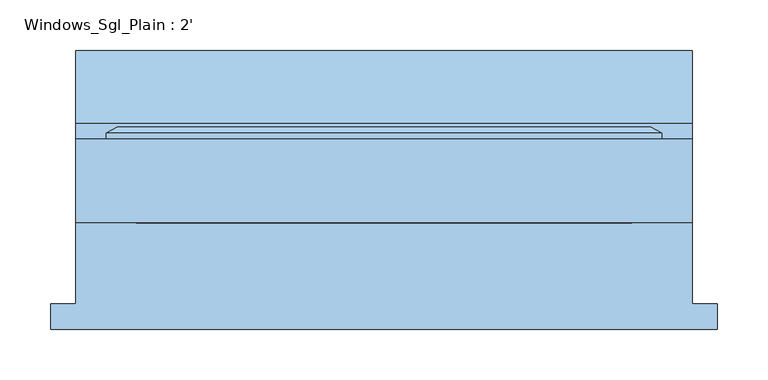
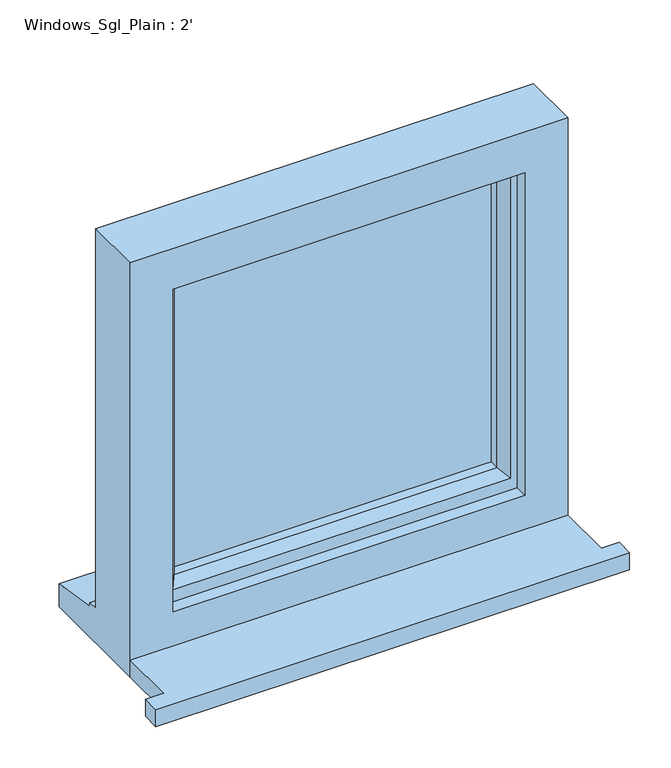
"""IFC4 building model written with IfcOpenShell, lengths in millimetres: window geometry, Windows_Sgl_Plain : 2'."""

from ifc_helpers import new_model, si_unit, frame, origin, place, context, project, spatial, polyline, outline, extrude, faceted_brep, source, transform, mapped, element, save


def windows_sgl_plain_2_298b83e7(model_context):
    return source(origin(), model_context, "Body", "SolidModel", [
        extrude(outline(polyline([(-329.8, -123.2234322), (-329.8, -98.2234322), (-304.8, -98.2234322), (-304.8, -17.8634322), (304.8, -17.8634322), (304.8, -98.2234322), (329.8, -98.2234322), (329.8, -123.2234322), (-329.8, -123.2234322)])), frame((0.0, 0.0, 1500.4), z_axis=(0.0, 0.0, 1.0), x_axis=(1.0, 0.0, 0.0)), (0.0, 0.0, 1.0), 25.0),
        faceted_brep([(-304.8, -17.8634322, 1500.4), (304.8, -17.8634322, 1500.4), (304.8, -17.8634322, 2110.0), (-304.8, -17.8634322, 2110.0), (-244.8, -17.8634322, 2050.0), (244.8, -17.8634322, 2050.0), (244.8, -17.8634322, 1575.4), (-244.8, -17.8634322, 1575.4), (-304.8, 65.1365678, 2110.0), (-304.8, 65.1365678, 1551.4), (-304.8, 80.1365678, 1550.08767), (-304.8, 80.1365678, 1545.1449676), (-304.8, 152.6365678, 1534.2088847), (-304.8, 152.6365678, 1500.4), (304.8, 65.1365678, 2110.0), (304.8, 65.1365678, 1551.4), (-264.8, 65.1365678, 2070.0), (-264.8, 65.1365678, 1563.4), (264.8, 65.1365678, 1563.4), (264.8, 65.1365678, 2070.0), (-264.8, 0.1365678, 2070.0), (-264.8, 0.1365678, 1563.4), (264.8, 0.1365678, 2070.0), (264.8, 0.1365678, 1563.4), (-244.8, 0.1365678, 2050.0), (-244.8, 0.1365678, 1575.4), (244.8, 0.1365678, 1575.4), (244.8, 0.1365678, 2050.0), (304.8, 152.6365678, 1500.4), (304.8, 152.6365678, 1534.2088847), (304.8, 80.1365678, 1545.1449676), (304.8, 80.1365678, 1550.08767)], [[[0, 1, 2, 3], [4, 5, 6, 7]], [[0, 3, 8, 9, 10, 11, 12, 13]], [[9, 8, 14, 15], [16, 17, 18, 19]], [[17, 16, 20, 21]], [[20, 22, 23, 21], [24, 25, 26, 27]], [[24, 4, 7, 25]], [[3, 2, 14, 8]], [[16, 19, 22, 20]], [[5, 4, 24, 27]], [[15, 14, 2, 1, 28, 29, 30, 31]], [[19, 18, 23, 22]], [[5, 27, 26, 6]], [[28, 1, 0, 13]], [[29, 28, 13, 12]], [[30, 29, 12, 11]], [[31, 30, 11, 10]], [[15, 31, 10, 9]], [[21, 23, 18, 17]], [[7, 6, 26, 25]]]),
        extrude(outline(polyline([(234.8, 29.1365678), (-234.8, 29.1365678), (-234.8, 53.1365678), (234.8, 53.1365678), (234.8, 29.1365678)])), frame((0.0, 0.0, 1593.4), z_axis=(0.0, 0.0, 1.0), x_axis=(1.0, 0.0, 0.0)), (0.0, 0.0, 1.0), 446.6),
        faceted_brep([(-274.8, 65.1365678, 2080.0), (-274.8, 70.9100705, 2080.0), (-274.8, 70.9100705, 1553.4), (-274.8, 65.1365678, 1553.4), (-264.8, 0.1365678, 2070.0), (-264.8, 65.1365678, 2070.0), (-264.8, 65.1365678, 1563.4), (-264.8, 0.1365678, 1563.4), (-224.8, 14.6294677, 2030.0), (-234.9480377, 0.1365678, 2040.1480377), (-234.9480377, 0.1365678, 1593.2519623), (-224.8, 14.6294677, 1603.4), (-224.8, 29.1365678, 2030.0), (-224.8, 29.1365678, 1603.4), (-234.8, 53.1365678, 2040.0), (-234.8, 29.1365678, 2040.0), (-234.8, 29.1365678, 1593.4), (-234.8, 53.1365678, 1593.4), (-224.8, 70.9100705, 2030.0), (-224.8, 53.1365678, 2030.0), (-224.8, 53.1365678, 1603.4), (-224.8, 70.9100705, 1603.4), (-242.2457548, 76.6835732, 2047.4457548), (-242.2457548, 76.6835732, 1585.9542452), (-264.0153903, 76.6835732, 2069.2153903), (-264.0153903, 76.6835732, 1564.1846097), (274.8, 70.9100705, 1553.4), (274.8, 65.1365678, 1553.4), (264.8, 65.1365678, 1563.4), (264.8, 0.1365678, 1563.4), (234.9480377, 0.1365678, 1593.2519623), (224.8, 14.6294677, 1603.4), (224.8, 29.1365678, 1603.4), (234.8, 29.1365678, 1593.4), (234.8, 53.1365678, 1593.4), (224.8, 53.1365678, 1603.4), (224.8, 70.9100705, 1603.4), (242.2457548, 76.6835732, 1585.9542452), (264.0153903, 76.6835732, 1564.1846097), (274.8, 70.9100705, 2080.0), (274.8, 65.1365678, 2080.0), (264.8, 65.1365678, 2070.0), (264.8, 0.1365678, 2070.0), (234.9480377, 0.1365678, 2040.1480377), (224.8, 14.6294677, 2030.0), (224.8, 29.1365678, 2030.0), (234.8, 29.1365678, 2040.0), (234.8, 53.1365678, 2040.0), (224.8, 53.1365678, 2030.0), (224.8, 70.9100705, 2030.0), (242.2457548, 76.6835732, 2047.4457548), (264.0153903, 76.6835732, 2069.2153903)], [[[0, 1, 2, 3]], [[4, 5, 6, 7]], [[8, 9, 10, 11]], [[12, 8, 11, 13]], [[14, 15, 16, 17]], [[18, 19, 20, 21]], [[22, 18, 21, 23]], [[1, 24, 25, 2]], [[3, 2, 26, 27]], [[7, 6, 28, 29]], [[11, 10, 30, 31]], [[13, 11, 31, 32]], [[17, 16, 33, 34]], [[21, 20, 35, 36]], [[23, 21, 36, 37]], [[2, 25, 38, 26]], [[27, 26, 39, 40]], [[29, 28, 41, 42]], [[31, 30, 43, 44]], [[32, 31, 44, 45]], [[34, 33, 46, 47]], [[36, 35, 48, 49]], [[37, 36, 49, 50]], [[26, 38, 51, 39]], [[40, 39, 1, 0]], [[3, 27, 40, 0], [5, 41, 28, 6]], [[42, 41, 5, 4]], [[7, 29, 42, 4], [9, 43, 30, 10]], [[44, 43, 9, 8]], [[45, 44, 8, 12]], [[15, 46, 33, 16], [13, 32, 45, 12]], [[47, 46, 15, 14]], [[17, 34, 47, 14], [19, 48, 35, 20]], [[49, 48, 19, 18]], [[50, 49, 18, 22]], [[24, 51, 38, 25], [23, 37, 50, 22]], [[39, 51, 24, 1]]]),
    ])


if __name__ == "__main__":
    model = new_model("IFC4")
    model_context = context("Model", 3, world=origin())
    ifc_project = project(units=[si_unit("LENGTHUNIT", "METRE", prefix="MILLI")], contexts=[model_context])
    site = spatial("IfcSite", under=ifc_project)
    building = spatial("IfcBuilding", under=site)
    placement = place(None, origin())
    windows_sgl_plain_2_shape = windows_sgl_plain_2_298b83e7(model_context)
    element("IfcWindow", 1, ObjectType="Windows_Sgl_Plain : 2'", at=placement, inside=building, context=model_context, shape_type="MappedRepresentation", body=[
        mapped(windows_sgl_plain_2_shape, transform((0.0, 0.0, 0.0), x_axis=(1.0, 0.0, 0.0), y_axis=(0.0, 1.0, 0.0), z_axis=(0.0, 0.0, 1.0))),
    ])
    save(model, "model.ifc")

# Revit data of these elements
# Type "Windows_Sgl_Plain : 2'"
#   Type Mark = "60"
#   Operation = "SinglePanel"
#   Construction Type Id = "SGL"
#   Manufacturer = "Revit"
#   Keynote = "L10"
#   Analytic Construction = "Large single-glazed windows"
#   Wrap Layers (Ext) from Ext = 0.336286 ft
#   Wrap Layers (Int) from Ext = 0.582349 ft
#   Window Board Projection = 0.082021 ft
#   Window Board Extension = 0.082021 ft
#   Visual Light Transmittance = 0.9
#   Solar Heat Gain Coefficient = 0.86
#   Rough Width = 2.0 ft
#   Rough Height = 2.0 ft
#   Height = 2.0 ft
#   Width = 2.0 ft
#   Heat Transfer Coefficient (U) = 5.5617 W/(m²·K)
#   Glazing Thickness = 0.07874 ft
#   FrameOffset - External = 0.164042 ft
#   Frame Depth = 0.213255 ft
#   Default Head Height = 6.922572 ft
#   Cill Depth = 0.287073 ft
#   Cavity Closer Width = 0.164042 ft
#   Cavity Closer Offset from Ext = 0.336286 ft
#   Cavity Closer Depth = 0.278871 ft
#   Vis - Cavity Closers = yes
#   Define Thermal Properties by = 1
#   Material Trim = Window Frame
#   Material Glass = Glass
#   Material Frame = Window Frame
#   Wall Closure = (empty or 0)
# Element 1 (IfcWindow, "Windows_Sgl_Plain : 2'")
#   Materials on its faces: "Window Frame", "Glass"
# Materials
#   "Window Frame": colour RGB 249 249 249, transparency 0, Keynote = "L10", Cost = 0
#   "Glass": class "Glass", colour RGB 0 128 192, transparency 0.9, Description = "Soda Lime Glass", Cost = 0
